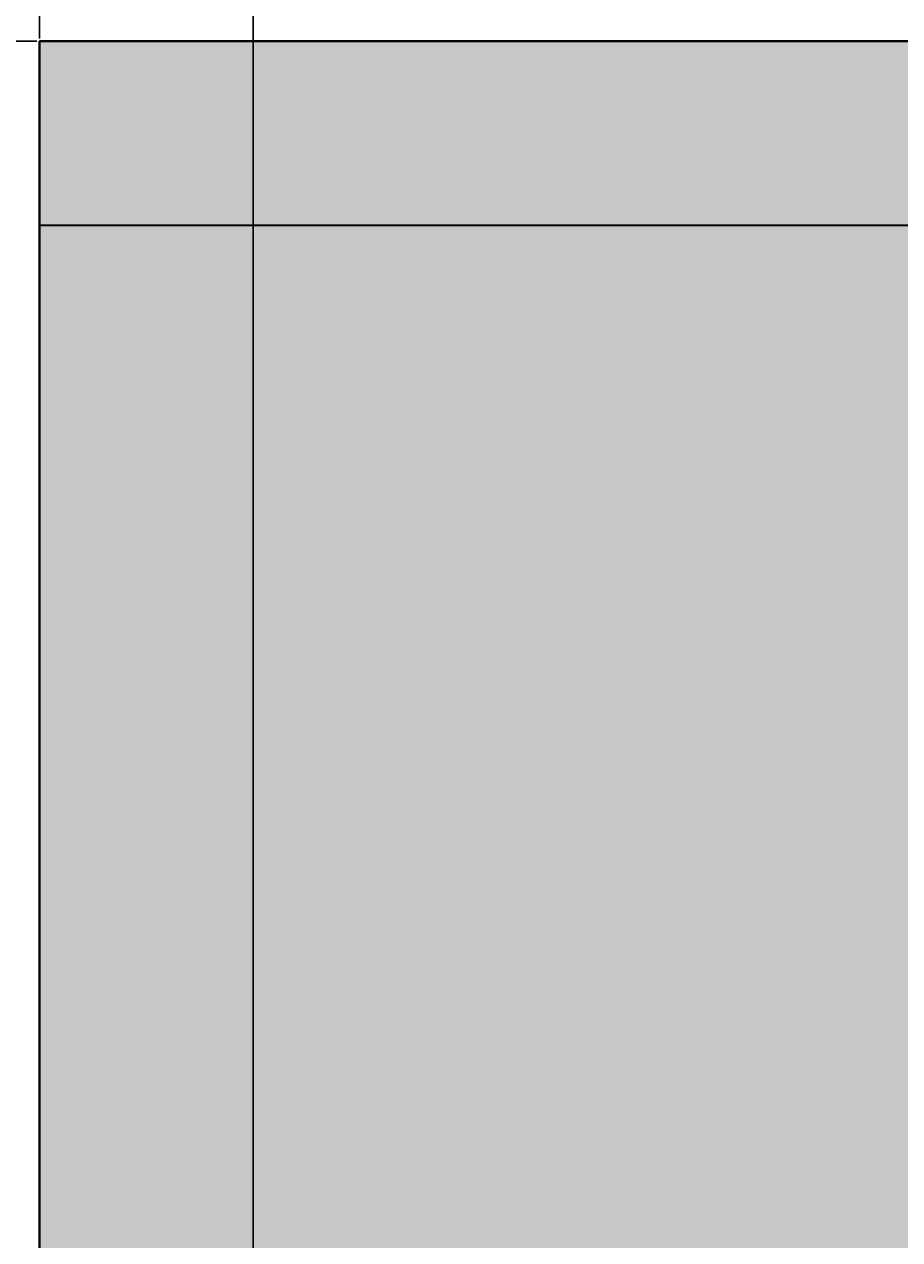
# Model space of a CAD drawing. Units: feet. Extents: x 2695 to 2912, y 795 to 1139.
# Tile 49 of 83: x 2710 to 2732, y 1093 to 1123. Entities that reach past the tile are written whole.
import ezdxf

# ---------------------------------------------------------------- set-up
doc = ezdxf.new("R2010")
doc.units = ezdxf.units.FT
for name, color, linetype, lineweight in [('A-ANNO-DIMS', 2, 'Continuous', 18), ('A-ELEV', 7, 'Continuous', 35), ('A-ELEV-PATT', 252, 'Continuous', 13)]:
    doc.layers.add(name, color=color, linetype=linetype, lineweight=lineweight)
doc.styles.get("Standard").update_dxf_attribs({"font": 'arial.ttf'})
doc.dimstyles.get("Standard").update_dxf_attribs({"dimtxt": 0.18, "dimasz": 0.18, "dimexe": 0.18, "dimexo": 0.0625, "dimgap": 0.09, "dimtad": 0, "dimtih": 1, "dimtoh": 1, "dimdec": 1, "dimzin": 0, "dimdsep": 46, "dimlunit": 3, "dimtxsty": 'Standard', "dimcen": 0.09, "dimadec": 0, "dimazin": 0, "dimtfac": 1, "dimtdec": 1, "dimtofl": 0, "dimtmove": 0, "dimatfit": 3, "dimfxl": 1, "dimtolj": 1, "dimtzin": 0, "dimarcsym": 0})

# ---------------------------------------------------------------- blocks, each defined once
blk = doc.blocks.new('*D7')
at = {"layer": 'A-ANNO-DIMS', "color": 0, "lineweight": -2, "transparency": 16777216}
for p, q in [((2710.636, 1122.993), (2710.636, 1138.886)), ((2710.816, 1138.706), (2712.867, 1138.706)), ((2715.705, 1138.706), (2713.655, 1138.706)), ((2715.885, 1050.373), (2715.885, 1138.886))]:
    blk.add_line(p, q, dxfattribs=at)
at = {"layer": 'A-ANNO-DIMS', "color": 0, "transparency": 16777216}
for points in [[(2710.816, 1138.736), (2710.816, 1138.676), (2710.636, 1138.706)], [(2715.705, 1138.736), (2715.705, 1138.676), (2715.885, 1138.706)]]:
    blk.add_solid(points, dxfattribs=at)
at = {"layer": 'Defpoints', "color": 0, "transparency": 16777216}
for p in [(2715.885, 1138.706), (2710.636, 1122.931), (2715.885, 1050.311)]:
    blk.add_point(p, dxfattribs=at)
at = {"layer": 'A-ANNO-DIMS', "color": 0, "transparency": 16777216, "insert": (2713.261, 1138.706), "char_height": 0.18, "attachment_point": 5}
blk.add_mtext('\\A1;5.249', dxfattribs=at)
blk = doc.blocks.new('*D8')
at = {"layer": 'A-ANNO-DIMS', "color": 0, "lineweight": -2, "transparency": 16777216}
for p, q in [((2715.885, 1050.373), (2715.885, 1138.886)), ((2716.065, 1138.706), (2742.866, 1138.706)), ((2770.456, 1138.706), (2743.655, 1138.706)), ((2770.636, 1122.993), (2770.636, 1138.886))]:
    blk.add_line(p, q, dxfattribs=at)
at = {"layer": 'A-ANNO-DIMS', "color": 0, "transparency": 16777216}
for points in [[(2716.065, 1138.736), (2716.065, 1138.676), (2715.885, 1138.706)], [(2770.456, 1138.736), (2770.456, 1138.676), (2770.636, 1138.706)]]:
    blk.add_solid(points, dxfattribs=at)
at = {"layer": 'Defpoints', "color": 0, "transparency": 16777216}
for p in [(2770.636, 1138.706), (2770.636, 1122.931), (2715.885, 1050.311)]:
    blk.add_point(p, dxfattribs=at)
at = {"layer": 'A-ANNO-DIMS', "color": 0, "transparency": 16777216, "insert": (2743.261, 1138.706), "char_height": 0.18, "attachment_point": 5}
blk.add_mtext('\\A1;54.75', dxfattribs=at)
blk = doc.blocks.new('*D12')
at = {"layer": 'A-ANNO-DIMS', "color": 0, "lineweight": -2, "transparency": 16777216}
for p, q in [((2710.574, 1122.931), (2694.681, 1122.931)), ((2694.861, 1122.751), (2694.861, 967.113)), ((2694.861, 811.111), (2694.861, 966.749)), ((2710.574, 810.931), (2694.681, 810.931))]:
    blk.add_line(p, q, dxfattribs=at)
at = {"layer": 'A-ANNO-DIMS', "color": 0, "transparency": 16777216}
for points in [[(2694.831, 1122.751), (2694.891, 1122.751), (2694.861, 1122.931)], [(2694.831, 811.111), (2694.891, 811.111), (2694.861, 810.931)]]:
    blk.add_solid(points, dxfattribs=at)
at = {"layer": 'Defpoints', "color": 0, "transparency": 16777216}
for p in [(2694.861, 1122.931), (2710.636, 1122.931), (2710.636, 810.931)]:
    blk.add_point(p, dxfattribs=at)
at = {"layer": 'A-ANNO-DIMS', "color": 0, "transparency": 16777216, "insert": (2694.861, 966.931), "char_height": 0.18, "attachment_point": 5}
blk.add_mtext('\\A1;312', dxfattribs=at)

msp = doc.modelspace()

# ---------------------------------------------------------------- hatches: boundary and pattern name
at = {"layer": 'A-ELEV-PATT'}
h = msp.add_hatch(color=256, dxfattribs=at)
h.set_gradient(color1=(255, 255, 255), tint=1)
h.paths.add_polyline_path([(2770.6361, 1122.9306), (2710.6361, 1122.9306), (2710.6361, 1118.4096), (2770.6361, 1118.4096)])
h.paths.add_polyline_path([(2890.6361, 1107.8588), (2770.6361, 1107.8588), (2770.6361, 1103.3378), (2890.6361, 1103.3378)])
h.paths.add_polyline_path([(2890.6361, 1062.9306), (2710.6361, 1062.9306), (2710.6361, 1056.9306), (2710.6361, 936.9306), (2710.6361, 924.3105), (2716.5358, 924.3105), (2890.6361, 924.3105), (2890.6361, 936.9306), (2715.8852, 936.9306), (2715.8852, 1050.3105), (2890.6361, 1050.3105)])
h.paths.add_polyline_path([(2716.5358, 924.3105), (2710.6361, 924.3105), (2710.6361, 810.9306), (2716.5358, 810.9306)])
h = msp.add_hatch(color=256, dxfattribs=at)
h.set_gradient(color1=(147, 149, 152), color2=(147, 149, 152), tint=1)
h.paths.add_polyline_path([(2770.6361, 1118.4096), (2710.6361, 1118.4096), (2710.6361, 1062.9306), (2770.6361, 1062.9306)])
h.paths.add_polyline_path([(2890.6361, 1103.3378), (2770.6361, 1103.3378), (2770.6361, 1062.9306), (2890.6361, 1062.9306)])
h.paths.add_polyline_path([(2730.7081, 1048.1052), (2755.1125, 1048.1052), (2755.1125, 936.9306), (2770.6361, 936.9306), (2770.6361, 1050.3105), (2715.8852, 1050.3105), (2715.8852, 936.9306), (2730.7081, 936.9306)])
h.paths.add_polyline_path([(2890.6361, 1050.3105), (2770.6361, 1050.3105), (2770.6361, 971.9673), (2778.0341, 971.9673), (2778.0341, 1020.8235), (2843.575, 1020.8235), (2843.575, 971.9673), (2890.6361, 971.9673)])
h.paths.add_polyline_path([(2888.1882, 970.7156), (2843.575, 970.7156), (2843.575, 964.8267), (2888.1882, 964.8267)])
h.paths.add_polyline_path([(2888.1882, 964.1328), (2843.575, 964.1328), (2843.575, 956.614), (2888.1882, 956.614)])
h.paths.add_polyline_path([(2888.1882, 955.9202), (2843.575, 955.9202), (2843.575, 949.2892), (2888.1882, 949.2892)])
h.paths.add_polyline_path([(2888.1882, 948.5954), (2843.575, 948.5954), (2843.575, 941.3507), (2888.1882, 941.3507)])
h.paths.add_polyline_path([(2888.1882, 940.6569), (2843.575, 940.6569), (2843.575, 936.9306), (2888.1882, 936.9306)])
h.paths.add_polyline_path([(2890.6361, 970.7156), (2888.9368, 970.7156), (2888.9368, 964.8267), (2890.6361, 964.8267)])
h.paths.add_polyline_path([(2890.6361, 964.1328), (2888.9368, 964.1328), (2888.9368, 956.614), (2890.6361, 956.614)])
h.paths.add_polyline_path([(2890.6361, 955.9202), (2888.9368, 955.9202), (2888.9368, 949.2892), (2890.6361, 949.2892)])
h.paths.add_polyline_path([(2890.6361, 940.6569), (2888.9368, 940.6569), (2888.9368, 936.9306), (2890.6361, 936.9306)])
h.paths.add_polyline_path([(2890.6361, 948.5954), (2888.9368, 948.5954), (2888.9368, 941.3507), (2890.6361, 941.3507)])
h.paths.add_polyline_path([(2772.5216, 970.7156), (2770.6361, 970.7156), (2770.6361, 964.8267), (2772.5216, 964.8267)])
h.paths.add_polyline_path([(2772.5216, 964.1328), (2770.6361, 964.1328), (2770.6361, 956.614), (2772.5216, 956.614)])
h.paths.add_polyline_path([(2772.5216, 955.9202), (2770.6361, 955.9202), (2770.6361, 949.2892), (2772.5216, 949.2892)])
h.paths.add_polyline_path([(2772.5216, 948.5954), (2770.6361, 948.5954), (2770.6361, 941.3507), (2772.5216, 941.3507)])
h.paths.add_polyline_path([(2772.5216, 940.6569), (2770.6361, 940.6569), (2770.6361, 936.9306), (2772.5216, 936.9306)])
h.paths.add_polyline_path([(2778.0341, 940.6569), (2773.2702, 940.6569), (2773.2702, 936.9306), (2778.0341, 936.9306)])
h.paths.add_polyline_path([(2778.0341, 970.7156), (2773.2702, 970.7156), (2773.2702, 964.8267), (2778.0341, 964.8267)])
h.paths.add_polyline_path([(2778.0341, 964.1328), (2773.2702, 964.1328), (2773.2702, 956.614), (2778.0341, 956.614)])
h.paths.add_polyline_path([(2778.0341, 955.9202), (2773.2702, 955.9202), (2773.2702, 949.2892), (2778.0341, 949.2892)])
h.paths.add_polyline_path([(2778.0341, 948.5954), (2773.2702, 948.5954), (2773.2702, 941.3507), (2778.0341, 941.3507)])
h.paths.add_polyline_path([(2810.0407, 940.6569), (2780.0341, 940.6569), (2780.0341, 936.9306), (2810.0407, 936.9306)])
h.paths.add_polyline_path([(2890.6361, 924.3105), (2770.6361, 924.3105), (2770.6361, 810.9306), (2773.5029, 810.9306), (2773.5029, 905.5143), (2805.9398, 905.5143), (2838.3767, 905.5143), (2838.3767, 810.9306), (2890.6361, 810.9306)])

# ---------------------------------------------------------------- linework, layer by layer
at = {"layer": 'A-ELEV'}
for p, q in [((2710.6361, 1062.9306), (2710.6361, 1122.9306)), ((2710.6361, 1122.9306), (2770.6361, 1122.9306)), ((2770.6361, 1122.9306), (2710.6361, 1122.9306)), ((2710.6361, 1122.9306), (2710.6361, 1118.4096)), ((2710.6361, 1118.4096), (2770.6361, 1118.4096)), ((2710.6361, 1118.4096), (2710.6361, 1062.9306))]:
    msp.add_line(p, q, dxfattribs=at)
msp.add_lwpolyline([(2710.6361, 1118.4096), (2770.6361, 1118.4096)], dxfattribs=at)

# ---------------------------------------------------------------- dimensions: what is measured, and where the dimension line sits
at = {"layer": 'A-ANNO-DIMS'}
for base, p1, p2, override, picture, middle in [((2715.8852, 1138.7056), (2710.6361, 1122.9306), (2715.8852, 1050.3105), {"dimdec": 3, "dimlfac": 1, "dimrnd": 0, "dimzin": 0, "dimdsep": 46, "dimlunit": 2}, '*D7', (2713.2606, 1138.7056)), ((2770.6361, 1138.7056), (2715.8852, 1050.3105), (2770.6361, 1122.9306), {"dimdec": 2, "dimlfac": 1, "dimrnd": 0, "dimzin": 0, "dimdsep": 46, "dimlunit": 2}, '*D8', (2743.2606, 1138.7056))]:
    dim = msp.add_linear_dim(base=base, p1=p1, p2=p2, dimstyle='Standard', override=override, dxfattribs=at)
    dim.commit()
    dim.dimension.update_dxf_attribs({"geometry": picture, "text_midpoint": middle})
dim = msp.add_linear_dim(base=(2694.8611, 1122.9306), p1=(2710.6361, 810.9306), p2=(2710.6361, 1122.9306), angle=90, dimstyle='Standard', override={"dimdec": 0, "dimlfac": 1, "dimrnd": 0, "dimzin": 0, "dimdsep": 46, "dimlunit": 2}, dxfattribs=at)
dim.commit()
dim.dimension.update_dxf_attribs({"geometry": '*D12', "text_midpoint": (2694.8611, 966.9306)})

doc.saveas('drawing.dxf')
